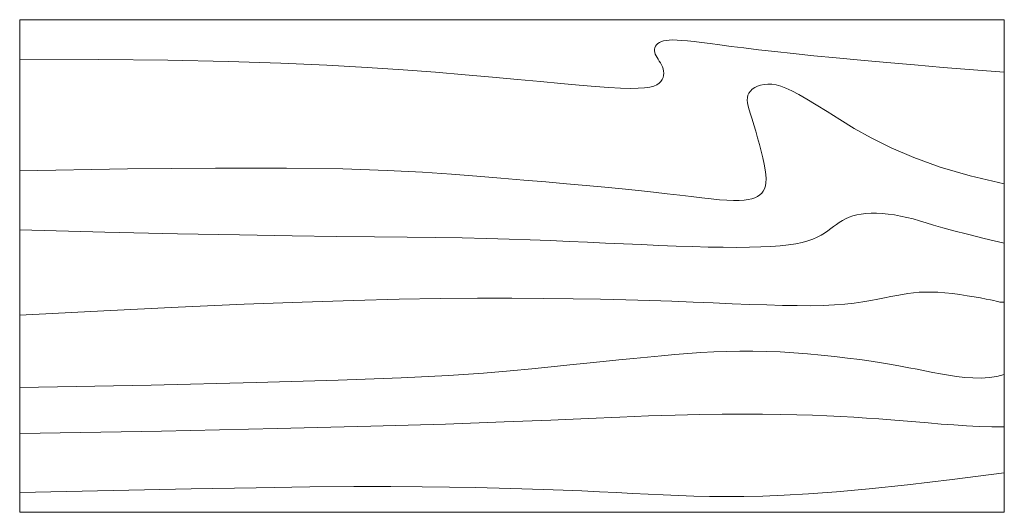
# Model space of a CAD drawing. Units: inches. Extents: x 821 to 2399, y 74 to 823.
# Tile 12 of 13: x 2279 to 2339, y 406 to 436. Entities that reach past the tile are written whole.
import ezdxf

# ---------------------------------------------------------------- set-up
doc = ezdxf.new("R2010")
doc.units = ezdxf.units.IN
doc.header["$MEASUREMENT"] = 0
doc.layers.get('0').update_dxf_attribs({"lineweight": 53})
doc.layers.add('A-FURN', color=8, linetype='Continuous', lineweight=18)

# ---------------------------------------------------------------- blocks, each defined once
blk = doc.blocks.new('Table - Rectangular Woodgrain 60 x 30 in.')
for p, q in [((0, 0), (0, -30)), ((60, 0), (0, 0)), ((60, -30), (60, 0)), ((0, -30), (60, -30))]:
    blk.add_line(p, q)
for points in [[(0, -2.4), (4.8155, -2.418), (9.0302, -2.4688), (12.709, -2.5477), (15.9167, -2.65), (18.7181, -2.7711), (21.1781, -2.9063), (23.3616, -3.0508), (25.3333, -3.2), (27.1477, -3.3495), (28.8172, -3.4958), (30.3437, -3.636), (31.7291, -3.7667), (32.9756, -3.8849), (34.0849, -3.9875), (35.059, -4.0714), (35.9, -4.1334), (36.6114, -4.1711), (37.2041, -4.1854), (37.6906, -4.1779), (38.0833, -4.15), (38.3948, -4.1034), (38.6375, -4.0396), (38.8239, -3.9602), (38.9666, -3.8667), (39.0764, -3.7608), (39.1573, -3.6448), (39.2116, -3.521), (39.2416, -3.3917), (39.2498, -3.2593), (39.2385, -3.1261), (39.21, -2.9944), (39.1666, -2.8667), (39.111, -2.7447), (39.0468, -2.6281), (38.978, -2.5163), (38.9083, -2.4083), (38.8418, -2.3035), (38.7823, -2.201), (38.7337, -2.1001), (38.7, -2), (38.6844, -1.9003), (38.6875, -1.8021), (38.7094, -1.707), (38.75, -1.6167), (38.8094, -1.5326), (38.8875, -1.4563), (38.9844, -1.3893), (39.1, -1.3333), (39.2351, -1.2896), (39.3937, -1.2583), (39.5804, -1.2396), (39.8, -1.2333), (40.057, -1.2396), (40.3562, -1.2583), (40.7023, -1.2896), (41.1, -1.3333), (41.5547, -1.3895), (42.0755, -1.4573), (42.6721, -1.5361), (43.3542, -1.625), (44.1316, -1.7233), (45.014, -1.8302), (46.0114, -1.9449), (47.1333, -2.0667), (48.3862, -2.1947), (49.7625, -2.3281), (51.2513, -2.4663), (52.8416, -2.6083), (54.5226, -2.7535), (56.2833, -2.9011), (58.1127, -3.0501), (60, -3.2)], [(0, -9.2), (6.5759, -9.0858), (11.9385, -9.0365), (16.2527, -9.0418), (19.6833, -9.0917), (22.3952, -9.1759), (24.5531, -9.2844), (26.322, -9.4069), (27.8666, -9.5333), (29.3241, -9.6553), (30.7203, -9.7719), (32.0532, -9.8837), (33.3208, -9.9917), (34.5213, -10.0965), (35.6526, -10.199), (36.7128, -10.2999), (37.7, -10.4), (38.6129, -10.4996), (39.4531, -10.5969), (40.223, -10.6895), (40.925, -10.775), (41.5613, -10.8512), (42.1344, -10.9156), (42.6465, -10.966), (43.1, -11), (43.4976, -11.0158), (43.8437, -11.0136), (44.143, -10.9942), (44.4, -10.9583), (44.6195, -10.9069), (44.8062, -10.8406), (44.9648, -10.7603), (45.1, -10.6667), (45.2155, -10.5598), (45.3114, -10.4365), (45.3871, -10.2929), (45.4416, -10.125), (45.4743, -9.929), (45.4844, -9.7011), (45.4709, -9.4371), (45.4333, -9.1333), (45.3716, -8.7883), (45.2896, -8.4104), (45.1919, -8.0107), (45.0833, -7.6), (44.9685, -7.1893), (44.8521, -6.7896), (44.7388, -6.4117), (44.6333, -6.0667), (44.54, -5.7628), (44.4614, -5.4979), (44.4001, -5.2675), (44.3583, -5.0667), (44.3384, -4.8909), (44.3427, -4.7354), (44.3736, -4.5956), (44.4333, -4.4667), (44.5236, -4.3453), (44.6427, -4.2333), (44.7884, -4.1339), (44.9583, -4.05), (45.1501, -3.9849), (45.3614, -3.9417), (45.59, -3.9234), (45.8333, -3.9333), (46.0915, -3.9749), (46.3734, -4.0531), (46.6906, -4.1736), (47.0542, -4.3417), (47.4756, -4.5629), (47.9661, -4.8427), (48.5372, -5.1866), (49.2, -5.6), (49.9676, -6.0844), (50.8594, -6.625), (51.8965, -7.2031), (53.1, -7.8), (54.491, -8.3969), (56.0906, -8.975), (57.9199, -9.5156), (60, -10)], [(0, -12.8), (5.1847, -12.9322), (9.6213, -13.0323), (13.3963, -13.1059), (16.5958, -13.1583), (19.3063, -13.1952), (21.614, -13.2219), (23.6054, -13.2439), (25.3666, -13.2667), (26.9728, -13.2947), (28.4531, -13.3281), (29.8256, -13.3663), (31.1083, -13.4083), (32.3191, -13.4535), (33.476, -13.501), (34.597, -13.5501), (35.7, -13.6), (36.7984, -13.6497), (37.8875, -13.6979), (38.9578, -13.743), (40, -13.7833), (41.0047, -13.8174), (41.9625, -13.8438), (42.864, -13.8607), (43.7, -13.8667), (44.4631, -13.8604), (45.1552, -13.8417), (45.7801, -13.8104), (46.3416, -13.7667), (46.8439, -13.7104), (47.2906, -13.6417), (47.6858, -13.5604), (48.0333, -13.4667), (48.3375, -13.3608), (48.6042, -13.2448), (48.8396, -13.121), (49.05, -12.9917), (49.2417, -12.8593), (49.4208, -12.7261), (49.5937, -12.5944), (49.7667, -12.4667), (49.9452, -12.3451), (50.1323, -12.2313), (50.3303, -12.1268), (50.5416, -12.0333), (50.7686, -11.9524), (51.0135, -11.8854), (51.2788, -11.8341), (51.5666, -11.8), (51.8785, -11.7843), (52.2116, -11.7865), (52.562, -11.8059), (52.926, -11.8417), (53.2998, -11.8931), (53.6795, -11.9594), (54.0614, -12.0397), (54.4416, -12.1333), (54.8223, -12.2401), (55.2293, -12.3625), (55.6942, -12.5037), (56.2489, -12.6667), (56.9251, -12.8547), (57.7545, -13.0708), (58.7689, -13.3182), (60, -13.6)], [(0, -18), (5.124, -17.7273), (9.6609, -17.5057), (13.6705, -17.3303), (17.2125, -17.1958), (20.3467, -17.0973), (23.1328, -17.0297), (25.6307, -16.9878), (27.9, -16.9667), (29.9928, -16.9617), (31.9302, -16.9703), (33.7254, -16.9907), (35.3917, -17.0208), (36.9423, -17.0588), (38.3906, -17.1026), (39.7499, -17.1503), (41.0333, -17.2), (42.2519, -17.2496), (43.4073, -17.2969), (44.4986, -17.3395), (45.525, -17.375), (46.4858, -17.4012), (47.3802, -17.4156), (48.2074, -17.416), (48.9667, -17.4), (49.6583, -17.3662), (50.2872, -17.3167), (50.8595, -17.2547), (51.3812, -17.1833), (51.8584, -17.1057), (52.2971, -17.025), (52.7034, -16.9443), (53.0833, -16.8667), (53.443, -16.7951), (53.789, -16.7313), (54.128, -16.6768), (54.4666, -16.6334), (54.8115, -16.6024), (55.1693, -16.5854), (55.5465, -16.5841), (55.95, -16.6), (56.3828, -16.6337), (56.8346, -16.6823), (57.2915, -16.7418), (57.7396, -16.8084), (58.165, -16.878), (58.5539, -16.9469), (58.8924, -17.0111), (59.1666, -17.0667), (59.3679, -17.1107), (59.5078, -17.1438), (59.6032, -17.1675), (59.6708, -17.1833), (59.7275, -17.193), (59.7901, -17.1979), (59.8753, -17.1998), (60, -17.2)], [(0, -22.4), (8.0098, -22.2501), (14.4094, -22.1011), (19.4168, -21.9535), (23.25, -21.8083), (26.1269, -21.6663), (28.2656, -21.5281), (29.884, -21.3947), (31.2, -21.2667), (32.3967, -21.1448), (33.5172, -21.0292), (34.5697, -20.9198), (35.5625, -20.8167), (36.5037, -20.7198), (37.4015, -20.6292), (38.2642, -20.5448), (39.1, -20.4667), (39.9164, -20.3951), (40.7187, -20.3313), (41.5117, -20.2768), (42.3, -20.2333), (43.0883, -20.2024), (43.8812, -20.1854), (44.6836, -20.1841), (45.5, -20.2), (46.3328, -20.234), (47.1747, -20.2844), (48.0163, -20.3488), (48.8479, -20.425), (49.66, -20.5106), (50.4429, -20.6031), (51.1872, -20.7004), (51.8833, -20.8), (52.5246, -20.8999), (53.1166, -20.9995), (53.6681, -21.0983), (54.1875, -21.1958), (54.6834, -21.2919), (55.1646, -21.3859), (55.6394, -21.4777), (56.1167, -21.5667), (56.6028, -21.6515), (57.0961, -21.7266), (57.5929, -21.7852), (58.0896, -21.8208), (58.5823, -21.8268), (59.0674, -21.7964), (59.5412, -21.723), (60, -21.6)], [(0, -25.2), (8.6355, -25.0504), (15.7026, -24.9031), (21.4049, -24.7606), (25.9458, -24.625), (29.529, -24.4988), (32.3578, -24.3844), (34.6359, -24.284), (36.5667, -24.2), (38.3213, -24.1341), (39.9417, -24.0854), (41.437, -24.0523), (42.8167, -24.0333), (44.0901, -24.0268), (45.2667, -24.0313), (46.3557, -24.0451), (47.3667, -24.0667), (48.309, -24.0947), (49.1928, -24.1287), (50.0284, -24.168), (50.826, -24.2125), (51.5959, -24.2617), (52.3483, -24.3151), (53.0935, -24.3725), (53.8417, -24.4334), (54.6009, -24.497), (55.3699, -24.561), (56.1454, -24.6226), (56.9239, -24.6792), (57.7021, -24.7279), (58.4764, -24.7662), (59.2435, -24.7911), (60, -24.8)], [(0, -28.8), (5.6867, -28.6681), (10.45, -28.5698), (14.407, -28.5012), (17.675, -28.4584), (20.3711, -28.4374), (22.6125, -28.4344), (24.5164, -28.4455), (26.2, -28.4667), (27.762, -28.4947), (29.2276, -28.5281), (30.6033, -28.5663), (31.8958, -28.6084), (33.1118, -28.6535), (34.2578, -28.7011), (35.3405, -28.7501), (36.3666, -28.8), (37.3443, -28.8497), (38.288, -28.8974), (39.2137, -28.9412), (40.1375, -28.9792), (41.0753, -29.0093), (42.0432, -29.0297), (43.0572, -29.0384), (44.1333, -29.0333), (45.2936, -29.0114), (46.5843, -28.9641), (48.0579, -28.8816), (49.7666, -28.7542), (51.7629, -28.5721), (54.0989, -28.3255), (56.8272, -28.0048), (60, -27.6)]]:
    blk.add_lwpolyline(points)

msp = doc.modelspace()

# ---------------------------------------------------------------- block references
at = {"layer": 'A-FURN'}
msp.add_blockref('Table - Rectangular Woodgrain 60 x 30 in.', (2279.173, 435.8106), dxfattribs=at)

doc.saveas('drawing.dxf')
